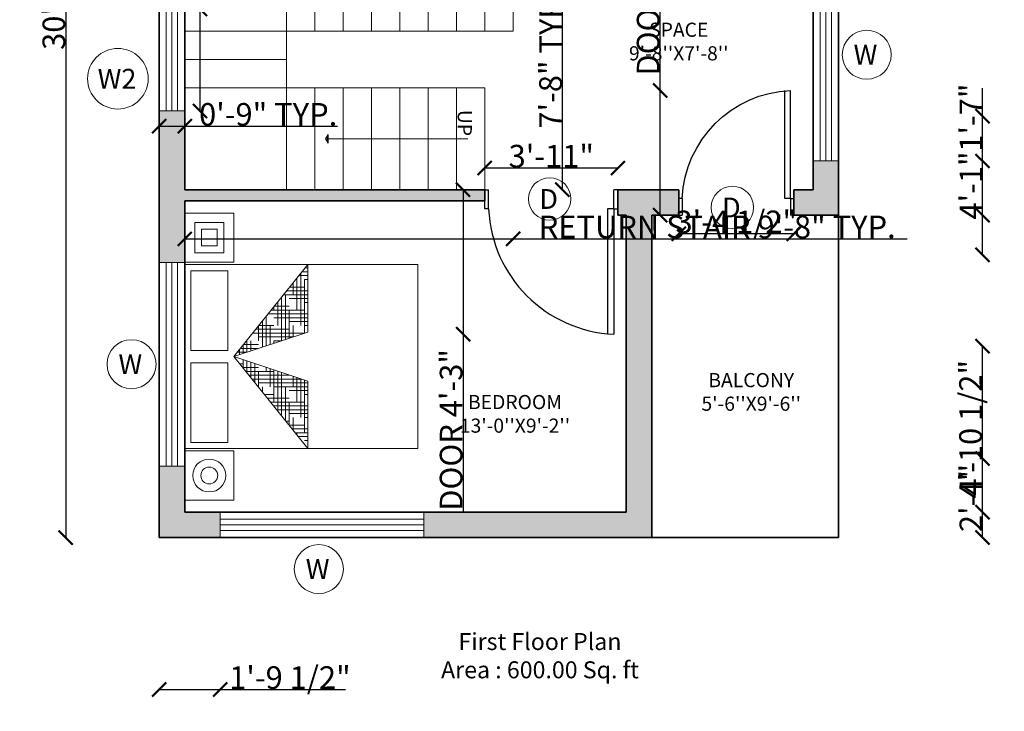
# Model space of a CAD drawing. Units: inches. Extents: x 2209 to 2954, y 1760 to 2265.
# Tile 5 of 7: x 2580 to 2928, y 1761 to 2005. Entities that reach past the tile are written whole.
import ezdxf

# ---------------------------------------------------------------- set-up
doc = ezdxf.new("R2010")
doc.units = ezdxf.units.IN
for name, color, linetype, lineweight in [('A-ANNO-DIMS', 2, 'Continuous', 18), ('A-ANNO-SYMB', 7, 'Continuous', 18), ('A-ANNO-TEXT', 7, 'Continuous', 25), ('A-AREA-IDEN', 7, 'Continuous', 18), ('A-FURN', 8, 'Continuous', 18), ('A-WALL-PATT', 30, 'Continuous', 13), ('DOOR', 240, 'Continuous', 25), ('STEPS', 50, 'Continuous', 18), ('WALL', 7, 'Continuous', 35), ('WINDOW', 190, 'Continuous', 18)]:
    doc.layers.add(name, color=color, linetype=linetype, lineweight=lineweight)
doc.styles.get("Standard").update_dxf_attribs({"font": 'arial.ttf'})
doc.dimstyles.get("Standard").update_dxf_attribs({"dimtxt": 8, "dimasz": 5, "dimexe": 0.18, "dimexo": 0.0625, "dimgap": 0.09, "dimtad": 1, "dimdec": 1, "dimzin": 0, "dimdsep": 46, "dimlunit": 4, "dimtxsty": 'Standard', "dimblk": 'ARCHTICK', "dimcen": 0.09, "dimse1": 1, "dimse2": 1, "dimadec": 0, "dimazin": 0, "dimtfac": 1, "dimtdec": 1, "dimtofl": 0, "dimtmove": 0, "dimatfit": 3, "dimfxl": 1, "dimtolj": 1, "dimtzin": 0, "dimarcsym": 0})

# ---------------------------------------------------------------- blocks, each defined once
blk = doc.blocks.new('AP0B05')
for p, q in [((35, 100), (35, 880)), ((75, 100), (75, 878.9)), ((35, 100), (11, 100)), ((11, 100), (11, -20)), ((35, 100), (35, -20)), ((815, 100), (815, -20)), ((815, 100), (839, 100)), ((839, 100), (839, -20)), ((11, -20), (35, -20)), ((839, -20), (815, -20))]:
    blk.add_line(p, q)
blk.add_lwpolyline([(35, 100), (75, 100)])
blk.add_arc((-2.4, 62.6), 818.3, 2.62122, 87.37878)
blk = doc.blocks.new('*X3')
at = {"color": 0}
for p, q in [((20.1875, 14.75), (20.1875, 14.7669)), ((20.199, 14.7812), (20.2772, 14.7812)), ((20.25, 14.8125), (20.2772, 14.8125)), ((20.1236, 14.6875), (20.25, 14.6875)), ((20.125, 14.5), (20.125, 14.6893)), ((20.1487, 14.7188), (20.2772, 14.7188)), ((20.1562, 14.625), (20.1562, 14.7281)), ((20.1739, 14.75), (20.2772, 14.75)), ((20.25, 14.3194), (20.25, 14.75)), ((20.0625, 14.2573), (20.0625, 14.6116)), ((20.0938, 14.375), (20.0938, 14.6504)), ((20.0984, 14.6562), (20.125, 14.6562)), ((20.2188, 14.3091), (20.2188, 14.625)), ((20.25, 14.625), (20.2772, 14.625)), ((19.9979, 14.5312), (20.2772, 14.5312)), ((20.023, 14.5625), (20.2772, 14.5625)), ((20.0312, 14.2469), (20.0312, 14.5727)), ((20.125, 14.5938), (20.2772, 14.5938)), ((19.9476, 14.4688), (20.125, 14.4688)), ((19.9727, 14.5), (20.25, 14.5)), ((20, 14.2366), (20, 14.5)), ((20.1875, 14.2987), (20.1875, 14.5)), ((19.875, 14.25), (19.875, 14.3785)), ((19.9062, 14.375), (19.9062, 14.4174)), ((19.9225, 14.4375), (20, 14.4375)), ((19.9688, 14.2262), (19.9688, 14.375)), ((20, 14.375), (20.2772, 14.375)), ((20.125, 14.4062), (20.2772, 14.4062)), ((20.1562, 14.2884), (20.1562, 14.375)), ((20.25, 14.4375), (20.2772, 14.4375)), ((19.7967, 14.2812), (20.125, 14.2812)), ((19.8125, 14.1744), (19.8125, 14.3008)), ((19.8219, 14.3125), (20.2291, 14.3125)), ((19.8438, 14.1848), (19.8438, 14.3397)), ((19.875, 14.3438), (20.2772, 14.3438)), ((19.7465, 14.2188), (19.875, 14.2188)), ((19.75, 14.1537), (19.75, 14.2231)), ((19.7716, 14.25), (20, 14.25)), ((19.7812, 14.1641), (19.7812, 14.262)), ((19.9375, 14.2159), (19.9375, 14.25)), ((19.7213, 14.1875), (19.75, 14.1875)), ((19.7018, 14.0938), (19.7786, 14.0938)), ((19.7188, 14.0726), (19.7188, 14.1136)), ((19.7269, 14.0625), (19.8728, 14.0625)), ((19.75, 14.0338), (19.75, 14.1032)), ((19.7812, 13.9949), (19.7812, 14.0929)), ((19.8125, 14), (19.8125, 14.0825)), ((19.9062, 13.8396), (19.9062, 14.0514)), ((19.9375, 13.8007), (19.9375, 14.0411)), ((19.752, 14.0312), (19.875, 14.0312)), ((19.875, 13.8784), (19.875, 14)), ((19.875, 13.9688), (20.1557, 13.9688)), ((19.9688, 13.875), (19.9688, 14.0307)), ((20, 14), (20, 14.0204)), ((20, 14), (20.0614, 14)), ((20.0625, 13.6454), (20.0625, 13.9996)), ((20.0938, 13.625), (20.0938, 13.9893)), ((20.125, 13.75), (20.125, 13.9789)), ((20.1562, 13.875), (20.1562, 13.9686)), ((19.8275, 13.9375), (20.25, 13.9375)), ((19.8526, 13.9062), (20.125, 13.9062)), ((20.25, 13.5), (20.25, 13.9375)), ((19.8777, 13.875), (20, 13.875)), ((20, 13.8125), (20.2772, 13.8125)), ((20.0312, 13.6842), (20.0312, 13.875)), ((20.125, 13.8438), (20.2772, 13.8438)), ((20.2188, 13.4511), (20.2188, 13.875)), ((20.25, 13.875), (20.2772, 13.875)), ((19.9532, 13.7812), (20.2772, 13.7812)), ((19.9783, 13.75), (20.25, 13.75)), ((20, 13.723), (20, 13.75)), ((20.0035, 13.7188), (20.125, 13.7188)), ((20.1875, 13.49), (20.1875, 13.75)), ((20.125, 13.6562), (20.2772, 13.6562)), ((20.25, 13.6875), (20.2772, 13.6875)), ((20.0789, 13.625), (20.2772, 13.625)), ((20.104, 13.5938), (20.2772, 13.5938)), ((20.1292, 13.5625), (20.25, 13.5625)), ((20.1562, 13.5288), (20.1562, 13.625)), ((20.25, 13.5), (20.2772, 13.5)), ((20.2046, 13.4688), (20.2772, 13.4688)), ((20.2297, 13.4375), (20.2772, 13.4375)), ((20.2549, 13.4062), (20.2772, 13.4062))]:
    blk.add_line(p, q, dxfattribs=at)
blk = doc.blocks.new('MAT-P13')
for p, q in [((-1.17, 0), (-1.17, -0.4)), ((-1.17, 0), (-0.77, 0)), ((-0.77, 0), (-0.77, -0.4)), ((-0.75, 0), (0.75, 0)), ((-0.75, 0), (-0.75, -1.9)), ((0.75, 0), (0.75, -1.9)), ((0.77, 0), (1.17, 0)), ((0.77, 0), (0.77, -0.4)), ((1.17, 0), (1.17, -0.4)), ((-0.7, -0.05), (-0.7, -0.35)), ((-0.7, -0.05), (-0.05, -0.05)), ((-0.05, -0.35), (-0.05, -0.05)), ((0.05, -0.05), (0.7, -0.05)), ((0.05, -0.35), (0.05, -0.05)), ((0.7, -0.05), (0.7, -0.35)), ((-1.17, -0.4), (-0.77, -0.4)), ((-0.75, -1.0034), (0, -0.4)), ((0, -0.4), (-0.75, -1.0034)), ((-0.7, -0.35), (-0.05, -0.35)), ((0, -0.4), (-0.2, -1.0034)), ((0, -0.4), (0.2, -1.0034)), ((0, -0.4), (0.75, -1.0034)), ((0.05, -0.35), (0.7, -0.35)), ((0.77, -0.4), (1.17, -0.4)), ((-0.75, -1.0034), (-0.2, -1.0034)), ((0.2, -1.0034), (0.75, -1.0034)), ((0.75, -1.9), (-0.75, -1.9))]:
    blk.add_line(p, q)
for points in [[(0.8468, -0.0814), (1.0932, -0.0814), (1.0932, -0.3186), (0.8468, -0.3186)], [(0.9015, -0.1361), (1.0385, -0.1361), (1.0385, -0.2639), (0.9015, -0.2639)]]:
    blk.add_lwpolyline(points, close=True)
for radius in [0.1342, 0.0686]:
    blk.add_circle((-0.97, -0.2), radius)
at = {"xscale": -1, "rotation": 90}
blk.add_blockref('*X3', (14.1285, 19.2738), dxfattribs=at)
blk = doc.blocks.new('_ArchTick')
at = {"color": 0, "linetype": 'ByBlock', "const_width": 0.15}
blk.add_lwpolyline([(-0.5, -0.5), (0.5, 0.5)], dxfattribs=at)
blk = doc.blocks.new('*D16')
at = {"layer": 'A-ANNO-DIMS', "color": 0, "lineweight": -2, "transparency": 16777216}
blk.add_line((2596.18, 2182.29), (2596.18, 1822.29), dxfattribs=at)
at = {"layer": 'Defpoints', "color": 0, "transparency": 16777216}
for p in [(2629.22, 2182.29), (2596.18, 1822.29), (2629.22, 1822.29)]:
    blk.add_point(p, dxfattribs=at)
at = {"layer": 'A-ANNO-DIMS', "color": 0, "lineweight": -2, "transparency": 16777216, "xscale": 5, "yscale": 5, "zscale": 5}
for p, rotation in [((2596.18, 2182.29), 90), ((2596.18, 1822.29), 270)]:
    blk.add_blockref('_ArchTick', p, dxfattribs=dict(at, rotation=rotation))
at = {"layer": 'A-ANNO-DIMS', "color": 0, "transparency": 16777216, "insert": (2592, 2002.29), "char_height": 8, "attachment_point": 5, "rotation": 90}
blk.add_mtext("\\A1;30'", dxfattribs=at)
blk = doc.blocks.new('WIN-W-72IN')
for p, q in [((0, 6.5), (72, 6.5)), ((0, 4.5), (72, 4.5)), ((0, 2.5), (72, 2.5))]:
    blk.add_line(p, q)
blk.add_lwpolyline([(0, 9), (72, 9), (72, 0), (0, 0)], close=True)
blk = doc.blocks.new('WIN-W2-36IN')
for p, q in [((2.5, 0), (2.5, 36)), ((4.5, 0), (4.5, 36)), ((6.5, 0), (6.5, 36))]:
    blk.add_line(p, q)
blk.add_lwpolyline([(0, 0), (0, 36), (9, 36), (9, 0)], close=True)
blk = doc.blocks.new('STAIR-RETURN-36IN')
for p, q in [((36, 0), (36, 92)), ((46, 56), (46, 92)), ((56, 56), (56, 92)), ((66, 56), (66, 92)), ((76, 56), (76, 92)), ((86, 56), (86, 92)), ((96, 56), (96, 92)), ((106, 56), (106, 92)), ((116, 56), (116, 92)), ((116, 56), (0, 56)), ((36, 46), (0, 46)), ((106, 36), (0, 36)), ((46, 0), (46, 36)), ((56, 0), (56, 36)), ((66, 0), (66, 36)), ((76, 0), (76, 36)), ((86, 0), (86, 36)), ((96, 0), (96, 36)), ((106, 0), (106, 36))]:
    blk.add_line(p, q)
blk = doc.blocks.new('TAG-OPENING-W')
blk.add_circle((0, 0), 8.66)
blk.add_text('W', height=7).set_placement((-4.62, -3.5))
blk = doc.blocks.new('TAG-OPENING-W2')
blk.add_circle((0, 0), 10.71)
blk.add_text('W2', height=7).set_placement((-7.14, -3.51))
blk = doc.blocks.new('TAG-OPENING-D')
blk.add_circle((0, 0), 7.5)
blk.add_text('D', height=7).set_placement((-3.65, -3.5))
blk = doc.blocks.new('ARROW-STAIR-DIRECTION')
h = blk.add_hatch()
h.set_pattern_fill('ANGLE', color=256, angle=90)
h.set_pattern_definition([(90, (1948.154, -2410.884), (-6.985, 4e-16), [5.08, -1.905]), (180, (1948.154, -2410.884), (-9e-16, -6.985), [5.08, -1.905])])
h.paths.add_polyline_path([(0, 1.5), (1, 0), (1, 3)])
for p, q in [((0, 1.5), (1, 3)), ((0, 1.5), (1, 0)), ((1, 0), (1, 3)), ((50.28, 1.5), (1, 1.5))]:
    blk.add_line(p, q)
blk = doc.blocks.new('*D29')
at = {"layer": 'A-ANNO-DIMS', "color": 0, "lineweight": -2, "transparency": 16777216}
for p, q in [((2643.62, 2009.14), (2643.62, 2135.42)), ((2643.62, 1973.14), (2643.62, 2009.14))]:
    blk.add_line(p, q, dxfattribs=at)
at = {"layer": 'Defpoints', "color": 0, "transparency": 16777216}
for p in [(2638.22, 2009.14), (2643.62, 2009.14), (2638.22, 1973.14)]:
    blk.add_point(p, dxfattribs=at)
at = {"layer": 'A-ANNO-DIMS', "color": 0, "lineweight": -2, "transparency": 16777216, "xscale": 5, "yscale": 5, "zscale": 5}
for p, rotation in [((2643.62, 2009.14), 90), ((2643.62, 1973.14), 270)]:
    blk.add_blockref('_ArchTick', p, dxfattribs=dict(at, rotation=rotation))
at = {"layer": 'A-ANNO-DIMS', "color": 0, "transparency": 16777216, "insert": (2639.38, 2074.78), "char_height": 8, "attachment_point": 5, "rotation": 90}
blk.add_mtext('\\A1;WINDOW W2 3\'-0" TYP.', dxfattribs=at)
blk = doc.blocks.new('*D30')
at = {"layer": 'A-ANNO-DIMS', "color": 0, "lineweight": -2, "transparency": 16777216}
for p, q in [((2629.22, 1967.74), (2638.22, 1967.74)), ((2638.22, 1967.74), (2692.16, 1967.74))]:
    blk.add_line(p, q, dxfattribs=at)
at = {"layer": 'Defpoints', "color": 0, "transparency": 16777216}
for p in [(2629.22, 1973.14), (2638.22, 1973.14), (2638.22, 1967.74)]:
    blk.add_point(p, dxfattribs=at)
at = {"layer": 'A-ANNO-DIMS', "color": 0, "lineweight": -2, "transparency": 16777216, "xscale": 5, "yscale": 5, "zscale": 5, "rotation": 180}
blk.add_blockref('_ArchTick', (2629.22, 1967.74), dxfattribs=at)
at = {"layer": 'A-ANNO-DIMS', "color": 0, "lineweight": -2, "transparency": 16777216, "xscale": 5, "yscale": 5, "zscale": 5}
blk.add_blockref('_ArchTick', (2638.22, 1967.74), dxfattribs=at)
at = {"layer": 'A-ANNO-DIMS', "color": 0, "transparency": 16777216, "insert": (2667.69, 1971.91), "char_height": 8, "attachment_point": 5}
blk.add_mtext('\\A1;0\'-9" TYP.', dxfattribs=at)
blk = doc.blocks.new('*D35')
at = {"layer": 'A-ANNO-DIMS', "color": 0, "lineweight": -2, "transparency": 16777216}
for p, q in [((2736.55, 1945.29), (2736.55, 1894.2)), ((2736.55, 1894.2), (2736.55, 1831.52))]:
    blk.add_line(p, q, dxfattribs=at)
at = {"layer": 'Defpoints', "color": 0, "transparency": 16777216}
for p in [(2744.22, 1945.29), (2736.55, 1894.2), (2744.22, 1894.2)]:
    blk.add_point(p, dxfattribs=at)
at = {"layer": 'A-ANNO-DIMS', "color": 0, "lineweight": -2, "transparency": 16777216, "xscale": 5, "yscale": 5, "zscale": 5}
for p, rotation in [((2736.55, 1945.29), 90), ((2736.55, 1894.2), 270)]:
    blk.add_blockref('_ArchTick', p, dxfattribs=dict(at, rotation=rotation))
at = {"layer": 'A-ANNO-DIMS', "color": 0, "transparency": 16777216, "insert": (2732.32, 1860.36), "char_height": 8, "attachment_point": 5, "rotation": 90}
blk.add_mtext('\\A1;DOOR 4\'-3"', dxfattribs=at)
blk = doc.blocks.new('*D36')
at = {"layer": 'A-ANNO-DIMS', "color": 0, "lineweight": -2, "transparency": 16777216}
blk.add_line((2791.22, 1952.95), (2744.22, 1952.95), dxfattribs=at)
at = {"layer": 'Defpoints', "color": 0, "transparency": 16777216}
for p in [(2744.22, 1952.95), (2744.22, 1945.29), (2791.22, 1945.29)]:
    blk.add_point(p, dxfattribs=at)
at = {"layer": 'A-ANNO-DIMS', "color": 0, "lineweight": -2, "transparency": 16777216, "xscale": 5, "yscale": 5, "zscale": 5, "rotation": 180}
blk.add_blockref('_ArchTick', (2744.22, 1952.95), dxfattribs=at)
at = {"layer": 'A-ANNO-DIMS', "color": 0, "lineweight": -2, "transparency": 16777216, "xscale": 5, "yscale": 5, "zscale": 5}
blk.add_blockref('_ArchTick', (2791.22, 1952.95), dxfattribs=at)
at = {"layer": 'A-ANNO-DIMS', "color": 0, "transparency": 16777216, "insert": (2767.72, 1957.13), "char_height": 8, "attachment_point": 5}
blk.add_mtext('\\A1;3\'-11"', dxfattribs=at)
blk = doc.blocks.new('*D39')
at = {"layer": 'A-ANNO-DIMS', "color": 0, "lineweight": -2, "transparency": 16777216}
for p, q in [((2806.16, 1980.39), (2806.16, 2043.07)), ((2806.16, 1936.29), (2806.16, 1980.39))]:
    blk.add_line(p, q, dxfattribs=at)
at = {"layer": 'Defpoints', "color": 0, "transparency": 16777216}
for p in [(2806.16, 1980.39), (2812.78, 1980.39), (2812.78, 1936.29)]:
    blk.add_point(p, dxfattribs=at)
at = {"layer": 'A-ANNO-DIMS', "color": 0, "lineweight": -2, "transparency": 16777216, "xscale": 5, "yscale": 5, "zscale": 5}
for p, rotation in [((2806.16, 1980.39), 90), ((2806.16, 1936.29), 270)]:
    blk.add_blockref('_ArchTick', p, dxfattribs=dict(at, rotation=rotation))
at = {"layer": 'A-ANNO-DIMS', "color": 0, "transparency": 16777216, "insert": (2801.93, 2014.23), "char_height": 8, "attachment_point": 5, "rotation": 90}
blk.add_mtext('\\A1;DOOR 3\'-8"', dxfattribs=at)
blk = doc.blocks.new('*D40')
at = {"layer": 'A-ANNO-DIMS', "color": 0, "lineweight": -2, "transparency": 16777216}
blk.add_line((2853.36, 1929.67), (2812.78, 1929.67), dxfattribs=at)
at = {"layer": 'Defpoints', "color": 0, "transparency": 16777216}
for p in [(2812.78, 1936.29), (2853.36, 1936.29), (2812.78, 1929.67)]:
    blk.add_point(p, dxfattribs=at)
at = {"layer": 'A-ANNO-DIMS', "color": 0, "lineweight": -2, "transparency": 16777216, "xscale": 5, "yscale": 5, "zscale": 5, "rotation": 180}
blk.add_blockref('_ArchTick', (2812.78, 1929.67), dxfattribs=at)
at = {"layer": 'A-ANNO-DIMS', "color": 0, "lineweight": -2, "transparency": 16777216, "xscale": 5, "yscale": 5, "zscale": 5}
blk.add_blockref('_ArchTick', (2853.36, 1929.67), dxfattribs=at)
at = {"layer": 'A-ANNO-DIMS', "color": 0, "transparency": 16777216, "insert": (2833.07, 1933.9), "char_height": 8, "attachment_point": 5}
blk.add_mtext('\\A1;3\'-4 1/2"', dxfattribs=at)
blk = doc.blocks.new('*D51')
at = {"layer": 'A-ANNO-DIMS', "color": 0, "lineweight": -2, "transparency": 16777216}
for p, q in [((2638.22, 1927.89), (2754.22, 1927.89)), ((2754.22, 1927.89), (2893.43, 1927.89))]:
    blk.add_line(p, q, dxfattribs=at)
at = {"layer": 'Defpoints', "color": 0, "transparency": 16777216}
for p in [(2638.22, 1945.29), (2754.22, 1945.29), (2754.22, 1927.89)]:
    blk.add_point(p, dxfattribs=at)
at = {"layer": 'A-ANNO-DIMS', "color": 0, "lineweight": -2, "transparency": 16777216, "xscale": 5, "yscale": 5, "zscale": 5, "rotation": 180}
blk.add_blockref('_ArchTick', (2638.22, 1927.89), dxfattribs=at)
at = {"layer": 'A-ANNO-DIMS', "color": 0, "lineweight": -2, "transparency": 16777216, "xscale": 5, "yscale": 5, "zscale": 5}
blk.add_blockref('_ArchTick', (2754.22, 1927.89), dxfattribs=at)
at = {"layer": 'A-ANNO-DIMS', "color": 0, "transparency": 16777216, "insert": (2826.32, 1932.11), "char_height": 8, "attachment_point": 5}
blk.add_mtext('\\A1;RETURN STAIR 9\'-8" TYP.', dxfattribs=at)
blk = doc.blocks.new('*D52')
at = {"layer": 'A-ANNO-DIMS', "color": 0, "lineweight": -2, "transparency": 16777216}
blk.add_line((2771.62, 1945.29), (2771.62, 2037.29), dxfattribs=at)
at = {"layer": 'Defpoints', "color": 0, "transparency": 16777216}
for p in [(2754.22, 2037.29), (2771.62, 2037.29), (2754.22, 1945.29)]:
    blk.add_point(p, dxfattribs=at)
at = {"layer": 'A-ANNO-DIMS', "color": 0, "lineweight": -2, "transparency": 16777216, "xscale": 5, "yscale": 5, "zscale": 5}
for p, rotation in [((2771.62, 2037.29), 90), ((2771.62, 1945.29), 270)]:
    blk.add_blockref('_ArchTick', p, dxfattribs=dict(at, rotation=rotation))
at = {"layer": 'A-ANNO-DIMS', "color": 0, "transparency": 16777216, "insert": (2767.44, 1991.29), "char_height": 8, "attachment_point": 5, "rotation": 90}
blk.add_mtext('\\A1;7\'-8" TYP.', dxfattribs=at)
blk = doc.blocks.new('*D74')
at = {"layer": 'A-ANNO-DIMS', "color": 0, "lineweight": -2, "transparency": 16777216}
blk.add_line((2920.04, 1822.29), (2920.04, 1850.29), dxfattribs=at)
at = {"layer": 'Defpoints', "color": 0, "transparency": 16777216}
for p in [(2519.15, 1850.29), (2920.04, 1850.29), (2519.15, 1822.29)]:
    blk.add_point(p, dxfattribs=at)
at = {"layer": 'A-ANNO-DIMS', "color": 0, "lineweight": -2, "transparency": 16777216, "xscale": 5, "yscale": 5, "zscale": 5}
for p, rotation in [((2920.04, 1850.29), 90), ((2920.04, 1822.29), 270)]:
    blk.add_blockref('_ArchTick', p, dxfattribs=dict(at, rotation=rotation))
at = {"layer": 'A-ANNO-DIMS', "color": 0, "transparency": 16777216, "insert": (2915.94, 1836.29), "char_height": 8, "attachment_point": 5, "rotation": 90}
blk.add_mtext('\\A1;2\'-4"', dxfattribs=at)
blk = doc.blocks.new('*D75')
at = {"layer": 'A-ANNO-DIMS', "color": 0, "lineweight": -2, "transparency": 16777216}
blk.add_line((2920.04, 1922.29), (2920.04, 1971.25), dxfattribs=at)
at = {"layer": 'Defpoints', "color": 0, "transparency": 16777216}
for p in [(2519.15, 1971.25), (2920.04, 1971.25), (2519.15, 1922.29)]:
    blk.add_point(p, dxfattribs=at)
at = {"layer": 'A-ANNO-DIMS', "color": 0, "lineweight": -2, "transparency": 16777216, "xscale": 5, "yscale": 5, "zscale": 5}
for p, rotation in [((2920.04, 1971.25), 90), ((2920.04, 1922.29), 270)]:
    blk.add_blockref('_ArchTick', p, dxfattribs=dict(at, rotation=rotation))
at = {"layer": 'A-ANNO-DIMS', "color": 0, "transparency": 16777216, "insert": (2915.94, 1946.77), "char_height": 8, "attachment_point": 5, "rotation": 90}
blk.add_mtext('\\A1;4\'-1"', dxfattribs=at)
blk = doc.blocks.new('*D80')
at = {"layer": 'A-ANNO-DIMS', "color": 0, "lineweight": -2, "transparency": 16777216}
blk.add_line((2920.04, 1831.29), (2920.04, 1889.91), dxfattribs=at)
at = {"layer": 'Defpoints', "color": 0, "transparency": 16777216}
for p in [(2509.59, 1889.91), (2920.04, 1889.91), (2510.15, 1831.29)]:
    blk.add_point(p, dxfattribs=at)
at = {"layer": 'A-ANNO-DIMS', "color": 0, "lineweight": -2, "transparency": 16777216, "xscale": 5, "yscale": 5, "zscale": 5}
for p, rotation in [((2920.04, 1889.91), 90), ((2920.04, 1831.29), 270)]:
    blk.add_blockref('_ArchTick', p, dxfattribs=dict(at, rotation=rotation))
at = {"layer": 'A-ANNO-DIMS', "color": 0, "transparency": 16777216, "insert": (2915.82, 1860.6), "char_height": 8, "attachment_point": 5, "rotation": 90}
blk.add_mtext('\\A1;4\'-10 1/2"', dxfattribs=at)
blk = doc.blocks.new('*D85')
at = {"layer": 'A-ANNO-DIMS', "color": 0, "lineweight": -2, "transparency": 16777216}
for p, q in [((2629.22, 1768.57), (2650.72, 1768.57)), ((2650.72, 1768.57), (2695.05, 1768.57))]:
    blk.add_line(p, q, dxfattribs=at)
at = {"layer": 'Defpoints', "color": 0, "transparency": 16777216}
for p in [(2629.22, 1822.29), (2650.72, 1822.29), (2650.72, 1768.57)]:
    blk.add_point(p, dxfattribs=at)
at = {"layer": 'A-ANNO-DIMS', "color": 0, "lineweight": -2, "transparency": 16777216, "xscale": 5, "yscale": 5, "zscale": 5, "rotation": 180}
blk.add_blockref('_ArchTick', (2629.22, 1768.57), dxfattribs=at)
at = {"layer": 'A-ANNO-DIMS', "color": 0, "lineweight": -2, "transparency": 16777216, "xscale": 5, "yscale": 5, "zscale": 5}
blk.add_blockref('_ArchTick', (2650.72, 1768.57), dxfattribs=at)
at = {"layer": 'A-ANNO-DIMS', "color": 0, "transparency": 16777216, "insert": (2675.38, 1772.79), "char_height": 8, "attachment_point": 5}
blk.add_mtext('\\A1;1\'-9 1/2"', dxfattribs=at)
blk = doc.blocks.new('*D88')
at = {"layer": 'A-ANNO-DIMS', "color": 0, "lineweight": -2, "transparency": 16777216}
blk.add_line((2224.78, 1919.53), (2224.78, 1973.14), dxfattribs=at)
at = {"layer": 'Defpoints', "color": 0, "transparency": 16777216}
for p in [(2224.78, 1973.14), (2629.22, 1973.14), (2629.22, 1919.53)]:
    blk.add_point(p, dxfattribs=at)
at = {"layer": 'A-ANNO-DIMS', "color": 0, "lineweight": -2, "transparency": 16777216, "xscale": 5, "yscale": 5, "zscale": 5}
for p, rotation in [((2224.78, 1973.14), 90), ((2224.78, 1919.53), 270)]:
    blk.add_blockref('_ArchTick', p, dxfattribs=dict(at, rotation=rotation))
at = {"layer": 'A-ANNO-DIMS', "color": 0, "transparency": 16777216, "insert": (2220.55, 1946.34), "char_height": 8, "attachment_point": 5, "rotation": 90}
blk.add_mtext('\\A1;4\'-5 1/2"', dxfattribs=at)
blk = doc.blocks.new('*D90')
at = {"layer": 'A-ANNO-DIMS', "color": 0, "lineweight": -2, "transparency": 16777216}
for p, q in [((2920.04, 1955.43), (2920.04, 1981.13)), ((2920.04, 1936.29), (2920.04, 1955.43))]:
    blk.add_line(p, q, dxfattribs=at)
at = {"layer": 'Defpoints', "color": 0, "transparency": 16777216}
for p in [(2869.22, 1955.43), (2920.04, 1955.43), (2869.22, 1936.29)]:
    blk.add_point(p, dxfattribs=at)
at = {"layer": 'A-ANNO-DIMS', "color": 0, "lineweight": -2, "transparency": 16777216, "xscale": 5, "yscale": 5, "zscale": 5}
for p, rotation in [((2920.04, 1955.43), 90), ((2920.04, 1936.29), 270)]:
    blk.add_blockref('_ArchTick', p, dxfattribs=dict(at, rotation=rotation))
at = {"layer": 'A-ANNO-DIMS', "color": 0, "transparency": 16777216, "insert": (2915.94, 1970.78), "char_height": 8, "attachment_point": 5, "rotation": 90}
blk.add_mtext('\\A1;1\'-7"', dxfattribs=at)

msp = doc.modelspace()

# ---------------------------------------------------------------- hatches: boundary and pattern name
at = {"layer": 'A-WALL-PATT', "transparency": 33554585}
h = msp.add_hatch(color=256, dxfattribs=at)
h.dxf.hatch_style = 1
h.paths.add_polyline_path([(2519.15, 2182.29), (2402.15, 2182.29), (2402.15, 2173.29), (2444.15, 2173.29), (2444.15, 2154.12), (2448.15, 2154.12), (2448.15, 2173.29), (2510.15, 2173.29), (2510.15, 2167.29), (2519.15, 2167.29)])
h.paths.add_polyline_path([(2330.15, 2182.29), (2279.15, 2182.29), (2279.15, 2145.83), (2288.15, 2145.83), (2288.15, 2158.01), (2288.15, 2173.29), (2330.15, 2173.29)])
h.paths.add_polyline_path([(2288.15, 2073.83), (2279.15, 2073.83), (2279.15, 2009.29), (2288.15, 2009.29), (2288.15, 2037.29), (2404.15, 2037.29), (2404.15, 2041.29), (2288.15, 2041.29)])
h.paths.add_polyline_path([(2519.15, 2131.29), (2510.15, 2131.29), (2510.15, 2125.29), (2444.15, 2125.29), (2444.15, 2041.29), (2439.11, 2041.29), (2439.11, 2037.29), (2448.15, 2037.29), (2448.15, 2069.29), (2481.65, 2069.29), (2481.65, 2073.29), (2448.15, 2073.29), (2448.15, 2121.29), (2468.19, 2121.29), (2468.19, 2121.32), (2488.37, 2121.32), (2510.15, 2121.29), (2510.15, 2113.63), (2519.15, 2113.63)])
h.paths.add_polyline_path([(2519.15, 2077.63), (2510.15, 2077.63), (2510.15, 2073.32), (2510.17, 2073.32), (2510.15, 2069.19), (2510.15, 2043.25), (2519.15, 2043.25)], flags=17)
h.paths.add_polyline_path([(2519.15, 1971.25), (2510.15, 1971.25), (2510.15, 1945.29), (2444.15, 1945.29), (2444.15, 1937.21), (2448.15, 1937.21), (2448.15, 1941.29), (2510.15, 1941.29), (2510.15, 1922.29), (2519.15, 1922.29)])
h.paths.add_polyline_path([(2288.15, 1941.29), (2394.15, 1941.29), (2394.15, 1945.29), (2288.15, 1945.29), (2288.15, 1973.29), (2279.15, 1973.29), (2279.15, 1919.97), (2288.15, 1919.97)])
h.paths.add_polyline_path([(2300.65, 1831.29), (2288.15, 1831.29), (2288.15, 1847.97), (2279.15, 1847.97), (2279.15, 1822.29), (2300.65, 1822.29)])
h.paths.add_polyline_path([(2394.15, 1825.29), (2394.15, 1831.29), (2372.65, 1831.29), (2372.65, 1822.29), (2394.15, 1822.29)])
h.paths.add_polyline_path([(2449.17, 1831.29), (2448.15, 1831.29), (2448.15, 1899.32), (2444.15, 1899.32), (2444.15, 1831.29), (2439.18, 1831.29), (2439.18, 1822.29), (2449.17, 1822.29)])
h.paths.add_polyline_path([(2519.15, 1850.29), (2510.15, 1850.29), (2510.15, 1831.29), (2509.17, 1831.29), (2509.17, 1822.29), (2519.15, 1822.29)])
h.paths.add_polyline_path([(2638.22, 1941.29), (2744.22, 1941.29), (2744.22, 1945.29), (2638.22, 1945.29), (2638.22, 1973.14), (2629.22, 1973.14), (2629.22, 1919.53), (2638.22, 1919.53)])
h.paths.add_polyline_path([(2638.22, 1847.53), (2629.22, 1847.53), (2629.22, 1822.29), (2650.72, 1822.29), (2650.72, 1831.29), (2638.22, 1831.29)])
h.paths.add_polyline_path([(2638.22, 2037.29), (2754.22, 2037.29), (2754.22, 2041.29), (2638.22, 2041.29), (2638.22, 2074.27), (2629.22, 2074.27), (2629.22, 2009.14), (2638.22, 2009.14)])
h.paths.add_polyline_path([(2803.22, 1936.29), (2812.78, 1936.29), (2812.78, 1945.29), (2791.22, 1945.29), (2791.22, 1936.29), (2794.22, 1936.29), (2794.22, 1831.29), (2722.72, 1831.29), (2722.72, 1822.29), (2803.22, 1822.29)])
h.paths.add_polyline_path([(2869.22, 1955.43), (2860.22, 1955.43), (2860.22, 1945.29), (2853.36, 1945.29), (2853.36, 1936.29), (2869.22, 1936.29)])
h.paths.add_polyline_path([(2680.22, 2182.29), (2629.22, 2182.29), (2629.22, 2146.27), (2638.22, 2146.27), (2638.22, 2173.29), (2680.22, 2173.29)])
h.paths.add_polyline_path([(2869.22, 2182.29), (2752.22, 2182.29), (2752.22, 2173.29), (2794.22, 2173.29), (2794.22, 2142.92), (2798.22, 2142.92), (2798.22, 2173.29), (2860.22, 2173.29), (2860.22, 2158.46), (2869.22, 2158.46)])
h.paths.add_polyline_path([(2869.22, 2122.46), (2860.22, 2122.46), (2860.22, 2090.29), (2869.22, 2090.29)])

# ---------------------------------------------------------------- linework, layer by layer
at = {"layer": 'WALL'}
for p, q in [((2629.22, 2182.29), (2629.22, 1822.29)), ((2869.22, 2182.29), (2869.22, 1822.29)), ((2638.22, 2037.29), (2638.22, 1945.29)), ((2860.22, 2037.29), (2860.22, 1945.29)), ((2638.22, 1945.29), (2744.22, 1945.29)), ((2744.22, 1945.29), (2744.22, 1941.29)), ((2812.78, 1945.29), (2791.22, 1945.29)), ((2791.22, 1945.29), (2791.22, 1936.29)), ((2812.78, 1945.29), (2812.78, 1936.29)), ((2853.36, 1945.29), (2853.36, 1936.29)), ((2853.36, 1945.29), (2860.22, 1945.29)), ((2638.22, 1941.29), (2638.22, 1831.29)), ((2638.22, 1941.29), (2744.22, 1941.29)), ((2791.22, 1936.29), (2794.22, 1936.29)), ((2794.22, 1936.29), (2794.22, 1831.29)), ((2803.22, 1936.29), (2803.22, 1822.29)), ((2803.22, 1936.29), (2812.78, 1936.29)), ((2853.36, 1936.29), (2869.22, 1936.29)), ((2638.22, 1831.29), (2794.22, 1831.29)), ((2629.22, 1822.29), (2869.22, 1822.29))]:
    msp.add_line(p, q, dxfattribs=at)

# ---------------------------------------------------------------- block references
at = {"layer": 'A-ANNO-SYMB'}
for name, p in [('TAG-OPENING-W', (2879.13, 1993.01)), ('TAG-OPENING-W2', (2614.61, 1984.52)), ('ARROW-STAIR-DIRECTION', (2687.93, 1961.79)), ('TAG-OPENING-D', (2767.14, 1942)), ('TAG-OPENING-D', (2831.7, 1939)), ('TAG-OPENING-W', (2619.43, 1883.58)), ('TAG-OPENING-W', (2685.6, 1811.16))]:
    msp.add_blockref(name, p, dxfattribs=at)
at = {"layer": 'A-FURN', "xscale": 43.35755422729858, "yscale": 43.35755422729858, "zscale": 43.35755422729858, "rotation": 90}
msp.add_blockref('MAT-P13', (2638.22, 1886.29), dxfattribs=at)
at = {"layer": 'DOOR', "xscale": -0.0490058245417994, "yscale": 0.0490058245417994, "zscale": 0.0490058245417994}
msp.add_blockref('AP0B05', (2853.9, 1937.27), dxfattribs=at)
at = {"layer": 'DOOR', "xscale": 0.0567632850241545, "yscale": 0.0567632850241545, "zscale": 0.0567632850241545, "rotation": 180}
msp.add_blockref('AP0B05', (2791.84, 1944.15), dxfattribs=at)
at = {"layer": 'STEPS'}
msp.add_blockref('STAIR-RETURN-36IN', (2638.21, 1945.29), dxfattribs=at)
at = {"layer": 'WINDOW'}
for p, rotation in [((2869.22, 1955.43), 89.99999999999972), ((2638.22, 1847.53), 89.99999999999962), ((2722.72, 1831.29), 180)]:
    msp.add_blockref('WIN-W-72IN', p, dxfattribs=dict(at, rotation=rotation))
msp.add_blockref('WIN-W2-36IN', (2629.21, 1973.14), dxfattribs=at)

# ---------------------------------------------------------------- texts
at = {"layer": 'A-ANNO-SYMB'}
msp.add_text('UP', height=5, rotation=270, dxfattribs=at).set_placement((2734.65, 1973.49))
at = {"layer": 'A-ANNO-TEXT', "insert": (2688.18, 1788.54), "char_height": 6, "attachment_point": 1}
msp.add_mtext_dynamic_manual_height_columns('\\pxqc;First Floor Plan\\PArea : 600.00 Sq. ft', width=151.0778, gutter_width=102.73, heights=[0], dxfattribs=at)
at = {"layer": 'A-AREA-IDEN', "char_height": 5, "attachment_point": 1}
for s, insert in [("\\pxqc;SPACE\\P9'-8''X7'-8''", (2790.17, 2004.33)), ("\\pxqc;BALCONY\\P5'-6''X9'-6''", (2815.78, 1880.46)), ("\\pxqc;BEDROOM\\P13'-0''X9'-2''", (2732.32, 1872.7))]:
    msp.add_mtext_dynamic_manual_height_columns(s, width=45.1409, gutter_width=12.5, heights=[0], dxfattribs=dict(at, insert=insert))

# ---------------------------------------------------------------- dimensions: what is measured, and where the dimension line sits
at = {"layer": 'A-ANNO-DIMS'}
for base, p1, p2, angle, override, picture, middle in [((2596.18, 1822.29), (2629.22, 2182.29), (2629.22, 1822.29), 90, {"dimclrd": 0, "dimclre": 0, "dimclrt": 0}, '*D16', (2592, 2002.29)), ((2920.04, 1955.43), (2869.22, 1936.29), (2869.22, 1955.43), 90, {"dimdec": 1, "dimlfac": 1, "dimrnd": 0, "dimzin": 1, "dimdsep": 46, "dimlunit": 4, "dimfrac": 2}, '*D90', (2915.94, 1970.78)), ((2224.78, 1973.14), (2629.22, 1919.53), (2629.22, 1973.14), 90, {"dimdec": 1, "dimlfac": 1, "dimrnd": 0, "dimzin": 1, "dimdsep": 46, "dimlunit": 4, "dimfrac": 2}, '*D88', (2220.55, 1946.34)), ((2920.04, 1971.25), (2519.15, 1922.29), (2519.15, 1971.25), 90, {"dimdec": 1, "dimlfac": 1, "dimrnd": 0, "dimzin": 1, "dimdsep": 46, "dimlunit": 4, "dimfrac": 2}, '*D75', (2915.94, 1946.77)), ((2744.22, 1952.95), (2791.22, 1945.29), (2744.22, 1945.29), 180, {"dimdec": 1, "dimlfac": 1, "dimrnd": 0, "dimzin": 1, "dimdsep": 46, "dimlunit": 4, "dimfrac": 2}, '*D36', (2767.72, 1957.13)), ((2812.78, 1929.67), (2853.36, 1936.29), (2812.78, 1936.29), 180, {"dimdec": 1, "dimlfac": 1, "dimrnd": 0, "dimzin": 1, "dimdsep": 46, "dimlunit": 4, "dimfrac": 2}, '*D40', (2833.07, 1933.9)), ((2920.04, 1889.91), (2510.15, 1831.29), (2509.59, 1889.91), 90, {"dimdec": 1, "dimlfac": 1, "dimrnd": 0, "dimzin": 1, "dimdsep": 46, "dimlunit": 4, "dimfrac": 2}, '*D80', (2915.82, 1860.6)), ((2920.04, 1850.29), (2519.15, 1822.29), (2519.15, 1850.29), 90, {"dimdec": 1, "dimlfac": 1, "dimrnd": 0, "dimzin": 1, "dimdsep": 46, "dimlunit": 4, "dimfrac": 2}, '*D74', (2915.94, 1836.29))]:
    dim = msp.add_linear_dim(base=base, p1=p1, p2=p2, angle=angle, dimstyle='Standard', override=override, dxfattribs=at)
    dim.commit()
    dim.dimension.update_dxf_attribs({"geometry": picture, "text_midpoint": middle})
for base, p1, p2, angle, text, picture, middle in [((2643.62, 2009.14), (2638.22, 1973.14), (2638.22, 2009.14), 90, 'WINDOW W2 <> TYP.', '*D29', (2639.38, 2074.78)), ((2806.16, 1980.39), (2812.78, 1936.29), (2812.78, 1980.39), 90, 'DOOR <>', '*D39', (2801.93, 2014.23)), ((2771.62, 2037.29), (2754.22, 1945.29), (2754.22, 2037.29), 90, '<> TYP.', '*D52', (2767.44, 1991.29)), ((2736.55, 1894.2), (2744.22, 1945.29), (2744.22, 1894.2), 270, 'DOOR <>', '*D35', (2732.32, 1860.36))]:
    dim = msp.add_linear_dim(base=base, p1=p1, p2=p2, angle=angle, text=text, dimstyle='Standard', override={"dimdec": 1, "dimlfac": 1, "dimrnd": 0, "dimzin": 1, "dimdsep": 46, "dimlunit": 4, "dimfrac": 2}, dxfattribs=at)
    dim.commit()
    dim.dimension.update_dxf_attribs({"geometry": picture, "text_midpoint": middle})
for base, p1, p2, text, picture, middle in [((2638.22, 1967.74), (2629.22, 1973.14), (2638.22, 1973.14), '<> TYP.', '*D30', (2667.69, 1971.91)), ((2754.22, 1927.89), (2638.22, 1945.29), (2754.22, 1945.29), 'RETURN STAIR <> TYP.', '*D51', (2826.32, 1932.11))]:
    dim = msp.add_linear_dim(base=base, p1=p1, p2=p2, text=text, dimstyle='Standard', override={"dimdec": 1, "dimlfac": 1, "dimrnd": 0, "dimzin": 1, "dimdsep": 46, "dimlunit": 4, "dimfrac": 2}, dxfattribs=at)
    dim.commit()
    dim.dimension.update_dxf_attribs({"geometry": picture, "text_midpoint": middle})
dim = msp.add_linear_dim(base=(2650.72, 1768.57), p1=(2629.22, 1822.29), p2=(2650.72, 1822.29), dimstyle='Standard', override={"dimdec": 1, "dimlfac": 1, "dimrnd": 0, "dimzin": 1, "dimdsep": 46, "dimlunit": 4, "dimfrac": 2}, dxfattribs=at)
dim.commit()
dim.dimension.update_dxf_attribs({"geometry": '*D85', "text_midpoint": (2675.38, 1772.79)})

doc.saveas('drawing.dxf')
